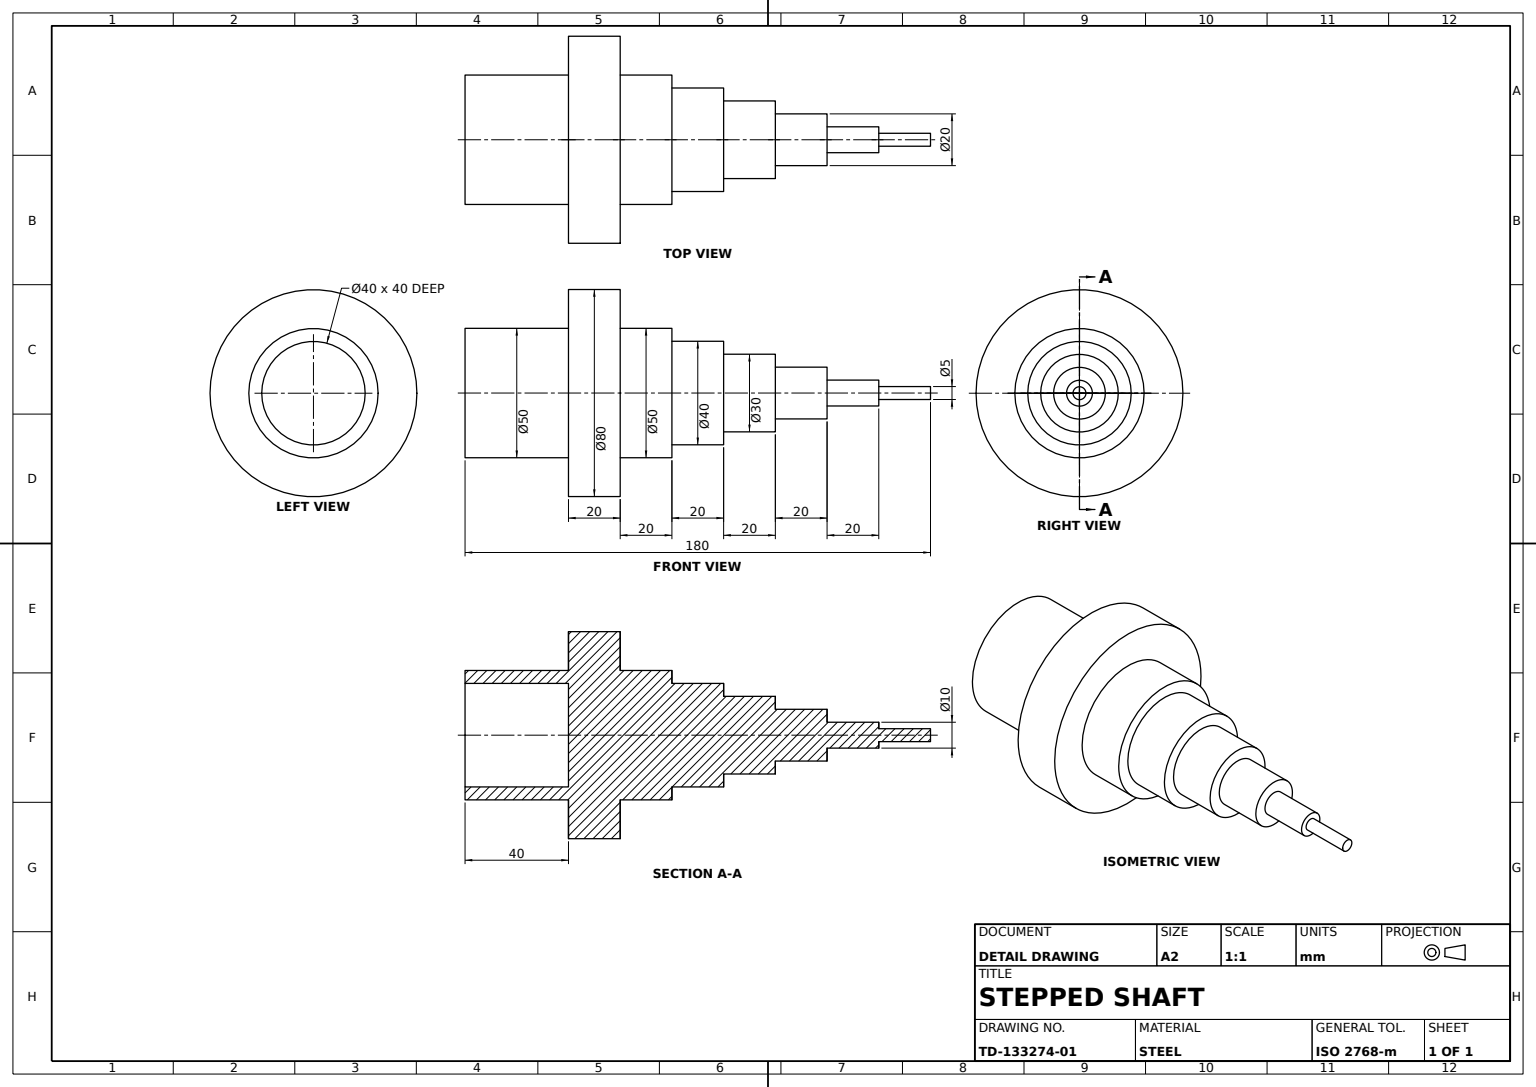
SolidWorks part; units mm, degrees
material "Plain Carbon Steel"
ref_plane "Front Plane" through (0, 0, 0) normal (0, 0, 1) x (1, 0, 0)
ref_plane "Top Plane" through (0, 0, 0) normal (0, 1, 0) x (1, 0, 0)
ref_plane "Right Plane" through (0, 0, 0) normal (1, 0, 0) x (0, 0, -1)
sketch "Shaft Profile Sketch" plane through (0, 0, 0) normal (0, 0, 1) x (1, 0, 0)
  line L0 (0, 50.2221) -> (0, -33.398) construction
  line L1 (-63.8507, 0) -> (144.247, 0) construction
  line L2 (-40, 0) -> (-40, 25)
  line L3 (-40, 25) -> (0, 25)
  line L4 (0, 25) -> (0, 40)
  line L5 (0, 40) -> (20, 40)
  line L6 (20, 40) -> (20, 25)
  line L7 (20, 25) -> (40, 25)
  line L8 (40, 25) -> (40, 20)
  line L9 (40, 20) -> (60, 20)
  line L10 (60, 20) -> (60, 15)
  line L11 (60, 15) -> (80, 15)
  line L12 (80, 15) -> (80, 10)
  line L13 (80, 10) -> (100, 10)
  line L14 (100, 10) -> (100, 5)
  line L15 (100, 5) -> (120, 5)
  line L16 (120, 5) -> (120, 2.5)
  line L17 (120, 2.5) -> (140, 2.5)
  line L18 (140, 2.5) -> (140, 0)
  line L19 (-40, 0) -> (140, 0)
  dimension "D1" = 40
  dimension "D2" = 25
  dimension "D3" = 15
  dimension "D4" = 20
  dimension "D5" = 25
  dimension "D6" = 20
  dimension "D7" = 20
  dimension "D8" = 20
  dimension "D9" = 15
  dimension "D10" = 20
  dimension "D11" = 10
  dimension "D12" = 20
  dimension "D13" = 20
  dimension "D14" = 2.5
  dimension "D15" = 20
  dimension "D16" = 2.5
revolve "Stepped Shaft Revolve" add sketch "Shaft Profile Sketch" angle 360 about L1
sketch "End Cut Sketch Ø40" plane through (-40, 0, 0) normal (-1, 0, 0) x (0, 0, 1)
  circle A0 centre (0, 0) radius 20
  dimension "D1" = 40
extrude "End Cut Ø40 x 40" cut sketch "End Cut Sketch Ø40" against normal blind 40
